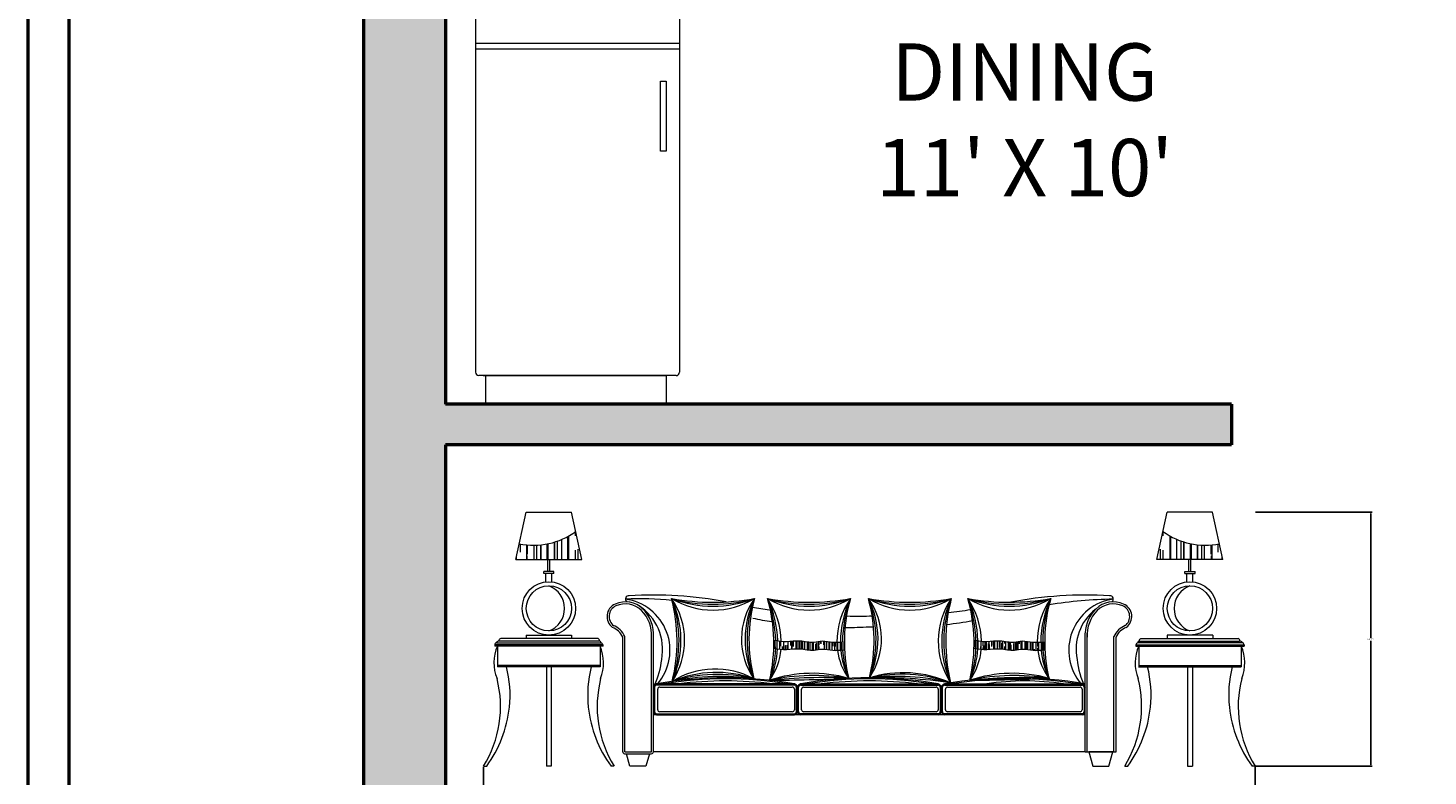
# Model space of a CAD drawing. Units: inches. Extents: x 1771 to 3025, y 319 to 889.
# Tile 31 of 35: x 2683 to 2854, y 714 to 805. Entities that reach past the tile are written whole.
import ezdxf

# ---------------------------------------------------------------- set-up
doc = ezdxf.new("R2010")
doc.units = ezdxf.units.IN
doc.header["$MEASUREMENT"] = 0
doc.set_wipeout_variables(frame=1)
for name, color, linetype, lineweight in [('A-ANNO-DIMS', 2, 'Continuous', 18), ('A-AREA-IDEN', 241, 'Continuous', 25), ('A-FURN', 8, 'Continuous', 18), ('A-WALL', 7, 'Continuous', 50), ('A-WALL-PATT', 254, 'Continuous', 13)]:
    doc.layers.add(name, color=color, linetype=linetype, lineweight=lineweight)
doc.styles.get("Standard").update_dxf_attribs({"font": 'arial.ttf'})
doc.dimstyles.get("Standard").update_dxf_attribs({"dimtxt": 0.18, "dimasz": 0.18, "dimexe": 0.18, "dimexo": 0.0625, "dimgap": 0.09, "dimtad": 0, "dimtih": 1, "dimtoh": 1, "dimdec": 4, "dimzin": 0, "dimdsep": 46, "dimtxsty": 'Standard', "dimcen": 0.09, "dimadec": 0, "dimazin": 0, "dimtfac": 1, "dimtdec": 4, "dimtofl": 0, "dimtmove": 0, "dimatfit": 3, "dimfxl": 1, "dimtolj": 1, "dimtzin": 0, "dimarcsym": 0})

# ---------------------------------------------------------------- blocks, each defined once
blk = doc.blocks.new('A$C301F3DA3')
for p, q in [((156.7, 1006), (206.7, 1236)), ((206.7, 1236), (427.8, 1236)), ((477.8, 1006), (427.8, 1236)), ((3275.4, 1006), (3325.4, 1236)), ((3546.5, 1236), (3325.4, 1236)), ((3596.5, 1006), (3546.5, 1236)), ((344.5, 1006), (344.5, 1090.3)), ((347, 1006), (347, 1091.1)), ((359.5, 1006), (359.5, 1095.2)), ((380.5, 1006), (380.5, 1103.5)), ((409.5, 1006), (409.5, 1117.6)), ((411, 1006), (411, 1118.4)), ((414, 1006), (414, 1120.1)), ((447.5, 1121.4), (447.5, 1141.6)), ((3305.7, 1121.4), (3305.7, 1141.6)), ((3339.2, 1006), (3339.2, 1120.1)), ((3342.2, 1006), (3342.2, 1118.4)), ((3343.7, 1006), (3343.7, 1117.6)), ((3372.7, 1006), (3372.7, 1103.5)), ((3393.7, 1006), (3393.7, 1095.2)), ((3406.2, 1006), (3406.2, 1091.1)), ((3408.7, 1006), (3408.7, 1090.3)), ((179.5, 1041.4), (179.5, 1081.1)), ((209.5, 1006), (209.5, 1076.8)), ((211.5, 1060.9), (211.5, 1076.6)), ((211.5, 1006), (211.5, 1023.4)), ((213, 1031.4), (213, 1076.5)), ((246.5, 1006), (246.5, 1075.2)), ((259.5, 1006), (259.5, 1075.6)), ((278, 1006), (278, 1073.4)), ((280, 1006), (280, 1077.1)), ((309.5, 1006), (309.5, 1081.6)), ((313.5, 1006), (313.5, 1082.4)), ((447.5, 1006), (447.5, 1051.4)), ((459.5, 1006), (459.5, 1056.4)), ((3293.7, 1006), (3293.7, 1056.4)), ((3305.7, 1006), (3305.7, 1051.4)), ((3439.7, 1006), (3439.7, 1082.4)), ((3443.7, 1006), (3443.7, 1081.6)), ((3473.2, 1006), (3473.2, 1077.1)), ((3475.2, 1006), (3475.2, 1073.4)), ((3493.7, 1006), (3493.7, 1075.6)), ((3506.7, 1006), (3506.7, 1075.2)), ((3540.2, 1031.4), (3540.2, 1076.5)), ((3541.7, 1060.9), (3541.7, 1076.6)), ((3541.7, 1006), (3541.7, 1023.4)), ((3543.7, 1006), (3543.7, 1076.8)), ((3573.7, 1041.4), (3573.7, 1081.1)), ((156.7, 1006), (477.8, 1006)), ((159.5, 1006), (159.5, 1019)), ((312.2, 948), (312.2, 1006)), ((322.2, 948), (322.2, 1006)), ((322.2, 948), (322.2, 1006)), ((477.5, 1006), (477.5, 1007.2)), ((3596.5, 1006), (3275.4, 1006)), ((3275.7, 1006), (3275.7, 1007.2)), ((3431, 948), (3431, 1006)), ((3431, 948), (3431, 1006)), ((3441, 948), (3441, 1006)), ((3593.7, 1006), (3593.7, 1019)), ((292.2, 938), (292.2, 948)), ((342.2, 948), (292.2, 948)), ((342.2, 938), (292.2, 938)), ((302.2, 896.9), (302.2, 938)), ((332.2, 896.9), (332.2, 938)), ((342.2, 938), (342.2, 948)), ((3411, 938), (3411, 948)), ((3411, 948), (3461, 948)), ((3411, 938), (3461, 938)), ((3421, 896.9), (3421, 938)), ((3451, 896.9), (3451, 938)), ((3461, 938), (3461, 948)), ((557.5, 620.8), (82.9, 620.8)), ((206.3, 637.8), (428.1, 637.8)), ((206.3, 637.8), (206.3, 620.8)), ((428.1, 637.8), (428.1, 620.8)), ((3195.6, 620.8), (3670.3, 620.8)), ((3546.9, 637.8), (3325, 637.8)), ((3325, 637.8), (3325, 620.8)), ((3546.9, 637.8), (3546.9, 620.8)), ((53.7, 590.8), (53.7, 584.4)), ((67.1, 584.4), (67.1, 484)), ((565.7, 608.8), (75.3, 608.8)), ((557.5, 608.8), (82.9, 608.8)), ((3187.5, 608.8), (3677.9, 608.8)), ((3195.6, 608.8), (3670.3, 608.8)), ((3686.1, 584.4), (3686.1, 484)), ((3699.5, 590.8), (3699.5, 584.4)), ((305.2, 484), (305.2, 0)), ((329.2, 484), (329.2, 0)), ((3424, 484), (3424, 0)), ((3448, 484), (3448, 0)), ((0, 0), (14.7, 0)), ((329.2, 0), (305.2, 0)), ((3424, 0), (3448, 0)), ((3753.2, 0), (3738.4, 0))]:
    blk.add_line(p, q)
for centre, radius in [((317.2, 767.8), 130), ((3436, 767.8), 130), ((317.2, 767.8), 110), ((3436, 767.8), 110)]:
    blk.add_circle(centre, radius)
for centre, radius, start, end in [((243.2, 1422.6), 347.4, 258.38286, 306.14668), ((3510, 1422.6), 347.4, 233.85332, 281.61714), ((276.7, 767.8), 117.2, 290.217, 69.783), ((3476.5, 767.8), 117.2, 110.217, 249.783), ((86.1, 609.2), 12.1, 105.22692, 181.3736), ((551.7, 609.3), 12.5, 357.63421, 66.98041), ((3201.5, 609.3), 12.5, 113.01959, 182.36579), ((3667.1, 609.2), 12.1, 358.6264, 74.77308), ((250.8, 503.3), 200.8, 156.16528, 202.38219), ((63.8, 591), 10.1, 100.6467, 181.11305), ((74, 595.7), 13.1, 84.28738, 156.7847), ((3679.2, 595.7), 13.1, 23.2153, 95.71262), ((3502.4, 503.3), 200.8, 337.61781, 23.83472), ((3689.4, 591), 10.1, 358.88695, 79.3533), ((-428.9, 346.4), 557.3, 353.82498, 14.29835), ((1063.3, 346.4), 557.3, 165.70165, 186.17502), ((2689.9, 346.4), 557.3, 353.82498, 14.29835), ((4182.1, 346.4), 557.3, 165.70165, 186.17502), ((-472, 290.4), 554.2, 328.39652, 14.25331), ((4225.2, 290.4), 554.2, 165.74669, 211.60348), ((-467.1, 350.3), 595.7, 323.98153, 353.84466), ((4220.2, 350.3), 595.7, 186.15534, 216.01847)]:
    blk.add_arc(centre, radius, start, end)
blk.add_wipeout([(3041.8, 0), (2963.5, 0), (2943.5, 70), (826.6, 70), (824.2, 65.5), (819.2, 61.4), (815.3, 60), (806.8, 60), (789.7, 0), (711.4, 0), (694.3, 60), (685.4, 60), (681.9, 61.7), (678.1, 65.9), (676.6, 70), (676.6, 628.7), (667.5, 644), (650.9, 661.4), (635.1, 671.5), (625.4, 676.3), (610.1, 693.4), (602.5, 710.5), (600.1, 728.4), (604.2, 751.4), (623, 778.5), (639.5, 788.9), (669, 798), (689.6, 799.7), (696.6, 800), (691.2, 806.8), (690.2, 814.9), (693.8, 823.2), (701.1, 828), (705.9, 828.8), (865.5, 832), (984.1, 825.9), (1111.6, 811), (1170.7, 801.2), (1180.3, 799.4), (1231.4, 803.5), (1293.2, 811.6), (1317.6, 815.8), (1310.3, 786.3), (1307.6, 774.2), (1389.8, 761.2), (1393.6, 767.5), (1388.1, 790.9), (1381.5, 815.8), (1418.2, 809.7), (1480.9, 802.2), (1546.1, 798.2), (1588.9, 797.6), (1683.4, 802), (1730, 807.2), (1784.7, 815.8), (1774.6, 776.7), (1767.8, 744), (1769.2, 730.8), (1890.2, 730.7), (1884.7, 761.4), (1877, 795.8), (1871.7, 815.8), (1919.1, 808.2), (1966.4, 802.7), (2026, 798.6), (2073.3, 797.6), (2145.9, 799.9), (2221.5, 807.4), (2273.8, 815.4), (2267.3, 783.6), (2260.5, 748.2), (2369.1, 762), (2361.7, 794), (2355.9, 815.8), (2402.1, 808.4), (2442.8, 803.5), (2477.3, 800.5), (2535.4, 797.9), (2572.4, 797.9), (2610.4, 806.1), (2648.6, 812), (2670.2, 815.1), (2740.7, 823.3), (2819.6, 829.3), (2905.4, 832.2), (2981.5, 831.5), (3045.3, 828.6), (3053.9, 827.3), (3059.6, 822.9), (3062.8, 816.3), (3062.9, 810.1), (3060.6, 804.3), (3056.6, 800), (3070.6, 799.5), (3085.9, 797.7), (3105.1, 792.4), (3120.7, 785.3), (3134.4, 774.5), (3143.7, 762.3), (3150.7, 746.2), (3153, 725.9), (3150.1, 708.7), (3142.9, 693.1), (3133.2, 681), (3126.6, 675.3), (3114.9, 669.8), (3100.2, 659.6), (3082.1, 638.7), (3076.6, 628.7), (3076.6, 70), (3061.8, 70)])
for p, q in [((3056.6, 800), (3056.6, 799.5)), ((676.6, 70), (676.6, 628.7)), ((686.6, 70), (686.6, 630.8)), ((816.6, 70), (816.6, 647.2)), ((826.6, 70), (826.6, 627.7)), ((2926.6, 70), (2926.6, 647.2)), ((2936.6, 70), (2936.6, 647.2)), ((3066.6, 70), (3066.6, 630.8)), ((3076.6, 70), (3076.6, 628.7)), ((580.7, 590.8), (53.7, 590.8)), ((580.7, 584.4), (53.7, 584.4)), ((61.9, 600.9), (572.5, 600.9)), ((566.3, 584.4), (566.3, 484)), ((579.7, 590.8), (579.7, 584.4)), ((3172.5, 590.8), (3699.5, 590.8)), ((3172.5, 584.4), (3699.5, 584.4)), ((3173.5, 590.8), (3173.5, 584.4)), ((3691.3, 600.9), (3180.7, 600.9)), ((3186.9, 584.4), (3186.9, 484)), ((567.3, 490), (67.1, 490)), ((567.3, 484), (67.1, 484)), ((3185.9, 490), (3686.1, 490)), ((3185.9, 484), (3686.1, 484)), ((826.6, 400), (826.6, 265)), ((1511.6, 400), (841.6, 400)), ((1511.2, 395), (841.6, 395)), ((846.6, 275), (846.6, 375)), ((856.6, 385), (1501.6, 385)), ((1511.6, 375), (1511.6, 275)), ((1526.6, 265), (1526.6, 385)), ((1526.6, 265), (1526.6, 385)), ((1531.6, 265.4), (1531.6, 384.6)), ((1541.6, 400), (2211.6, 400)), ((1542, 395), (2211.2, 395)), ((1546.6, 275), (1546.6, 375)), ((1556.6, 385), (2201.6, 385)), ((2211.6, 375), (2211.6, 275)), ((2221.6, 384.6), (2221.6, 265.4)), ((2226.6, 265), (2226.6, 385)), ((2226.6, 385), (2226.6, 265)), ((2231.6, 265.4), (2231.6, 384.6)), ((2241.6, 400), (2911.6, 400)), ((2242, 395), (2911.2, 395)), ((2246.6, 275), (2246.6, 375)), ((2256.6, 385), (2901.6, 385)), ((2911.6, 375), (2911.6, 275)), ((2921.6, 384.6), (2921.6, 265.4)), ((1511.6, 250), (826.6, 250)), ((2926.6, 250), (826.6, 250)), ((841.6, 250), (1511.6, 250)), ((842, 255), (1511.6, 255)), ((1501.6, 265), (856.6, 265)), ((2211.6, 255), (1542, 255)), ((2201.6, 265), (1556.6, 265)), ((2911.2, 255), (2242, 255)), ((2901.6, 265), (2256.6, 265)), ((686.6, 70), (816.6, 70)), ((2926.6, 70), (826.6, 70)), ((2926.6, 70), (3076.6, 70)), ((3061.8, 70), (2943.5, 70)), ((2943.5, 70), (2963.5, 0)), ((3041.8, 0), (3061.8, 70)), ((633.4, 0), (618.7, 0)), ((685.4, 60), (815.3, 60)), ((711.4, 0), (694.3, 60)), ((789.7, 0), (711.4, 0)), ((806.8, 60), (789.7, 0)), ((2963.5, 0), (3041.8, 0)), ((3119.8, 0), (3134.5, 0))]:
    blk.add_line(p, q)
at = {"ltscale": 0.1}
for p, q in [((1414.4, 573.7), (1414.4, 606.7)), ((1418.8, 573), (1418.8, 612.1)), ((1420.6, 572.7), (1420.6, 580.7)), ((1427.8, 571.6), (1427.8, 610.7)), ((1440.6, 576.7), (1440.6, 609)), ((1441.2, 569.8), (1441.2, 608.9)), ((1445.4, 583.3), (1445.4, 608.4)), ((1454.6, 568.5), (1454.6, 582.7)), ((1460.6, 568.1), (1460.6, 607.2)), ((1468, 606.7), (1468, 607)), ((1468, 567.8), (1468, 586.7)), ((1472, 603.3), (1472, 606.9)), ((1472, 567.8), (1472, 588.3)), ((1480.6, 568.1), (1480.6, 588.7)), ((1481.4, 568.1), (1481.4, 607.3)), ((1494.8, 586.7), (1494.8, 608.3)), ((1498.6, 569.5), (1498.6, 608.3)), ((1500.6, 569.7), (1500.6, 608.8)), ((1508.2, 582.7), (1508.2, 609.5)), ((1520.6, 571.3), (1520.6, 610.4)), ((1521.6, 571.4), (1521.6, 610.5)), ((1525.2, 571.5), (1525.2, 610.6)), ((1535, 571.6), (1535, 610.7)), ((1540.6, 571.3), (1540.6, 610.4)), ((1548.4, 570.6), (1548.4, 609.6)), ((1551.8, 570.1), (1551.8, 609.2)), ((1560.6, 568.8), (1560.6, 607.9)), ((1561.8, 568.6), (1561.8, 607.7)), ((1575.2, 566.4), (1575.2, 605.5)), ((1578.4, 565.9), (1578.4, 605)), ((1580.6, 565.6), (1580.6, 604.7)), ((1588.6, 564.6), (1588.6, 603.7)), ((1600.6, 564), (1600.6, 603.1)), ((1602, 564), (1602, 590.7)), ((1605, 568.3), (1605, 603.3)), ((1615.4, 565.2), (1615.4, 594.7)), ((1620.6, 566.1), (1620.6, 600.7)), ((1628.8, 567.7), (1628.8, 606.9)), ((1631.6, 588.3), (1631.6, 607.4)), ((1631.6, 568.2), (1631.6, 581.7)), ((1640.6, 596.7), (1640.6, 608.8)), ((1642.2, 594.7), (1642.2, 609)), ((1655.6, 590.7), (1655.6, 609.3)), ((1655.6, 570.2), (1655.6, 570.7)), ((1658.2, 608.3), (1658.2, 609.1)), ((1658.2, 570), (1658.2, 601.7)), ((1660.6, 569.8), (1660.6, 608.9)), ((1669, 568.8), (1669, 607.9)), ((1680.6, 566.9), (1680.6, 606)), ((1682.4, 570.7), (1682.4, 605.7)), ((1684.8, 566.2), (1684.8, 605.3)), ((1695.8, 566.7), (1695.8, 603.7)), ((1700.6, 584.7), (1700.6, 603.2)), ((1700.6, 564.1), (1700.6, 564.7)), ((1709.2, 563.6), (1709.2, 602.7)), ((1711.4, 581.7), (1711.4, 602.7)), ((1711.4, 563.6), (1711.4, 566.7)), ((1720.6, 563.7), (1720.6, 602.8)), ((1722.6, 563.7), (1722.6, 602.9)), ((1736, 564.6), (1736, 603.8)), ((1738, 601.7), (1738, 603.9)), ((1738, 564.8), (1738, 586.7)), ((1740.6, 565), (1740.6, 604.2)), ((1749.4, 565.9), (1749.4, 598.7)), ((2392.6, 573.1), (2392.6, 610.7)), ((2400.6, 571.9), (2400.6, 610.9)), ((2403, 571.5), (2403, 610.6)), ((2406, 571.1), (2406, 610.1)), ((2419.4, 569.4), (2419.4, 582.7)), ((2420.6, 569.2), (2420.6, 608.3)), ((2429.6, 583.5), (2429.6, 607.5)), ((2429.6, 568.4), (2429.6, 576.9)), ((2432.8, 606.7), (2432.8, 607.3)), ((2432.8, 568.2), (2432.8, 586.7)), ((2440.6, 567.9), (2440.6, 607)), ((2446.2, 567.8), (2446.2, 606.9)), ((2456.2, 603.5), (2456.2, 607.3)), ((2456.2, 568.1), (2456.2, 596.9)), ((2459.6, 586.7), (2459.6, 607.5)), ((2460.6, 568.4), (2460.6, 592.7)), ((2473, 582.7), (2473, 608.6)), ((2480.6, 588.7), (2480.6, 609.3)), ((2482.8, 570.4), (2482.8, 609.5)), ((2486.4, 570.7), (2486.4, 609.8)), ((2499.8, 571.5), (2499.8, 610.6)), ((2500.6, 571.5), (2500.6, 610.7)), ((2509.4, 576.9), (2509.4, 610.7)), ((2513.2, 571.4), (2513.2, 610.5)), ((2520.6, 570.8), (2520.6, 600.7)), ((2526.6, 570.1), (2526.6, 609.1)), ((2536, 596.9), (2536, 607.7)), ((2536, 568.6), (2536, 581.9)), ((2540, 568), (2540, 607)), ((2540.6, 576.7), (2540.6, 606.9)), ((2553.4, 565.8), (2553.4, 604.9)), ((2560.6, 564.9), (2560.6, 604)), ((2562.6, 564.7), (2562.6, 601.9)), ((2566.8, 564.3), (2566.8, 590.7)), ((2580.2, 564.2), (2580.2, 594.7)), ((2580.6, 564.2), (2580.6, 603.3)), ((2589.2, 565.2), (2589.2, 604.3)), ((2593.6, 565.9), (2593.6, 605.1)), ((2600.6, 567.2), (2600.6, 606.4)), ((2607, 594.7), (2607, 607.6)), ((2615.8, 569.8), (2615.8, 608.9)), ((2620.4, 590.7), (2620.4, 609.3)), ((2620.4, 570.2), (2620.4, 570.7)), ((2620.6, 570.2), (2620.6, 609.3)), ((2633.8, 570), (2633.8, 609)), ((2640.6, 569.2), (2640.6, 608.3)), ((2642.4, 569), (2642.4, 608)), ((2647.2, 570.7), (2647.2, 607.3)), ((2660.6, 566), (2660.6, 605.1)), ((2660.6, 566.7), (2660.6, 605.1)), ((2669, 564.8), (2669, 603.8)), ((2674, 564.2), (2674, 603.3)), ((2680.6, 563.8), (2680.6, 568.7)), ((2687.4, 563.6), (2687.4, 602.7)), ((2695.6, 581.9), (2695.6, 602.8)), ((2695.6, 563.7), (2695.6, 575.3)), ((2700.6, 564.7), (2700.6, 603.1)), ((2700.8, 563.9), (2700.8, 603.1)), ((2714.2, 565), (2714.2, 598.7)), ((2720.6, 565.6), (2720.6, 604.8)), ((2722.2, 601.9), (2722.2, 604.9)), ((2722.2, 565.8), (2722.2, 595.3)), ((2727.6, 566.4), (2727.6, 602.7))]:
    blk.add_line(p, q, dxfattribs=at)
at = {"ltscale": 0.2}
for p, q in [((831.6, 384.6), (831.6, 265.4)), ((1521.6, 265.4), (1521.6, 384.6))]:
    blk.add_line(p, q, dxfattribs=at)
for centre, radius, start, end in [((705.9, 812.9), 15.9, 82.92998, 233.99863), ((826.9, -1080.6), 1912.9, 79.35353, 93.56712), ((2926.5, -1083.7), 1916.1, 86.44665, 100.89711), ((3047.3, 812.9), 15.9, 306.00137, 97.07002), ((666.4, 728.4), 66.3, 113.9424, 233.11156), ((666.4, 728.4), 56.3, 113.9424, 233.11156), ((689.6, 677.8), 121.9, 45.5351, 114.26403), ((689.6, 677.8), 111.9, 45.5351, 114.26403), ((647.8, 638.7), 169.2, 356.50689, 44.75015), ((647.8, 638.7), 179.2, 356.50689, 44.75015), ((118.5, 608.8), 822.4, 346.1538, 14.5736), ((1116, 1923.3), 1125.7, 259.68325, 280.31675), ((2062.3, 614.6), 771.4, 164.88081, 194.22903), ((1820.4, 3753.3), 3022.9, 260.23295, 261.81056), ((611.7, 598.3), 800, 346.95646, 15.77378), ((1583.1, 1923.3), 1125.7, 259.68325, 280.31675), ((2517.6, 605.2), 762.6, 163.96966, 193.48898), ((2073.3, 1923.3), 1125.7, 259.68325, 280.31675), ((1147.1, 613.7), 752.3, 345.86352, 15.58525), ((3098.6, 604.6), 850.3, 165.62179, 193.5679), ((1932.8, 3753.3), 3022.9, 276.22345, 278.29852), ((2556.6, 1923.4), 1125.7, 259.73156, 280.36506), ((1586.1, 598.3), 800, 346.95646, 15.77378), ((3493.3, 605.3), 763.9, 163.98353, 193.47734), ((3105.4, 638.7), 179.2, 135.24985, 176.50689), ((3105.4, 638.7), 169.2, 135.24985, 183.49311), ((3063.6, 677.8), 121.9, 65.73597, 134.4649), ((3063.6, 677.8), 111.9, 65.73597, 134.4649), ((3086.8, 728.4), 56.3, 306.88844, 66.0576), ((3086.8, 728.4), 66.3, 306.88844, 66.0576), ((593.4, 589.7), 101.9, 23.83547, 68.81673), ((1820.4, 3753.3), 3022.9, 269.03014, 271.06523), ((1932.8, 3753.3), 3022.9, 268.93477, 269.19298), ((3159.8, 589.7), 101.9, 112.01062, 156.16453), ((593.4, 589.7), 91.9, 24.95202, 68.81673), ((3159.8, 589.7), 91.9, 111.18327, 155.04798), ((561.8, 599.3), 9.8, 9.61841, 76.53695), ((382.6, 503.3), 200.8, 337.61781, 23.83472), ((562.8, 585.5), 17.7, 17.55797, 60.68227), ((3370.5, 503.3), 200.8, 156.16528, 202.38219), ((3190.4, 585.5), 17.7, 119.31773, 162.44203), ((3191.3, 599.3), 9.8, 103.46305, 170.38159), ((1106.4, 290.4), 554.2, 165.74669, 211.60348), ((1176.6, -1455.4), 1885.4, 79.76537, 100.23463), ((1150.7, -658.8), 1096, 81.40397, 102.31547), ((1256.5, 13610.3), 13193.2, 270.58435, 272.25734), ((1876.6, -1455.4), 1885.4, 79.76537, 100.23463), ((1933.3, -1830.3), 2260.9, 81.38364, 91.43687), ((2584.1, -1540.1), 1970.1, 79.98833, 100.01167), ((2230.8, 13610.3), 13193.2, 270.58435, 272.25734), ((2646.8, 290.4), 554.2, 328.39652, 14.25331), ((844.1, 382.5), 17.7, 98.1301, 171.8699), ((844.1, 382.5), 12.7, 101.3731, 171.8699), ((856.6, 375), 10, 90, 180), ((1501.6, 375), 10, 0, 90), ((1509.1, 382.5), 12.7, 9.60357, 81.8699), ((1509.1, 382.5), 17.7, 8.1301, 81.8699), ((1544.1, 382.5), 17.7, 98.1301, 171.8699), ((1544.1, 382.5), 12.7, 99.60357, 170.39643), ((1556.6, 375), 10, 90, 180), ((2201.6, 375), 10, 0, 90), ((2209.1, 382.5), 12.7, 9.60357, 81.8699), ((2209.1, 382.5), 17.7, 8.1301, 81.8699), ((2244.1, 382.5), 17.7, 98.1301, 171.8699), ((2244.1, 382.5), 12.7, 98.1301, 170.39643), ((2256.6, 375), 10, 90, 180), ((2901.6, 375), 10, 0, 90), ((2909.1, 382.5), 12.7, 9.60357, 80.39643), ((2909.1, 382.5), 17.7, 8.1301, 81.8699), ((1101.5, 350.3), 595.7, 186.15534, 216.01847), ((856.6, 275), 10, 180, 270), ((1501.6, 275), 10, 270, 0), ((1556.6, 275), 10, 180, 270), ((2201.6, 275), 10, 270, 0), ((2256.6, 275), 10, 180, 270), ((2901.6, 275), 10, 270, 0), ((2651.7, 350.3), 595.7, 323.98153, 353.84466), ((844.1, 267.5), 17.7, 188.1301, 261.8699), ((844.1, 267.5), 12.7, 189.60357, 260.39643), ((1509.1, 267.5), 12.7, 278.1301, 351.8699), ((1509.1, 267.5), 17.7, 278.1301, 351.8699), ((1544.1, 267.5), 17.7, 188.1301, 261.8699), ((1544.1, 267.5), 12.7, 188.1301, 261.8699), ((2209.1, 267.5), 12.7, 278.1301, 350.39643), ((2209.1, 267.5), 17.7, 278.1301, 351.8699), ((2244.1, 267.5), 17.7, 188.1301, 261.8699), ((2244.1, 267.5), 12.7, 189.60357, 261.8699), ((2909.1, 267.5), 12.7, 278.1301, 350.39643), ((2909.1, 267.5), 17.7, 278.1301, 351.8699), ((689.4, 72.4), 13, 190.46913, 252.22973), ((812.4, 74.7), 15, 281.33001, 341.83756)]:
    blk.add_arc(centre, radius, start, end)
for centre, radius, start, end in [((760.4, -701.1), 1515.6, 84.07641, 92.659), ((655.5, 564.2), 251.1, 319.40416, 82.09148), ((615.4, 566.9), 255.3, 349.39262, 57.21951), ((478.9, 611.1), 481.1, 335.55638, 25.17102), ((347.1, 610.3), 603.3, 340.81637, 19.91104), ((617, 612), 360.5, 326.31194, 34.41547), ((1116, 1147.7), 388.4, 238.72737, 301.27263), ((1116, 1532.7), 744.8, 254.29016, 285.61296), ((1116.1, 1337.7), 559.4, 249.04787, 290.9906), ((1594, 618.2), 339.8, 144.44675, 214.66309), ((1723.9, 617.2), 452.3, 153.95498, 205.15486), ((1847.8, 616.2), 566.5, 159.37514, 199.7347), ((757.4, 589.8), 663.8, 1.89953, 19.9071), ((904.2, 593.4), 526.6, 1.83653, 24.977), ((1057.3, 597.5), 390.8, 1.55805, 33.94797), ((1583.1, 1147.7), 388.4, 238.72737, 301.27263), ((1583.2, 1532.7), 744.8, 254.29016, 285.61296), ((1583.2, 1337.7), 559.4, 249.04787, 290.9906), ((2089.5, 604.3), 371, 145.24271, 180.23552), ((2233.6, 600.8), 497.7, 154.4139, 179.66501), ((2371.5, 597.7), 626, 159.61394, 179.36153), ((2073.3, 1147.7), 388.4, 238.72737, 301.27263), ((2073.4, 1532.7), 744.8, 254.29016, 285.61296), ((1604, 619.4), 332, 325.19263, 36.25614), ((1356.4, 616.3), 552.6, 340.29034, 21.15843), ((1477.2, 617.8), 441.4, 334.80604, 26.64273), ((2073.4, 1337.7), 559.4, 249.04787, 290.9906), ((2583.5, 608.3), 371.9, 146.08399, 213.1057), ((2726, 607.2), 497, 155.19256, 203.99713), ((2862.3, 606.3), 623.6, 160.37041, 198.81928), ((2557.2, 1147.9), 388.4, 238.77569, 301.32093), ((1731.8, 589.8), 663.8, 1.89953, 19.9071), ((1878.6, 593.4), 526.6, 1.83653, 24.977), ((2031.7, 597.5), 390.8, 1.55805, 33.94797), ((2556.9, 1532.9), 744.8, 254.33859, 285.66141), ((2557.2, 1337.9), 559.4, 249.09653, 291.03924), ((3065, 604.3), 372, 145.29362, 180.23636), ((3209.5, 600.8), 499.2, 154.45299, 179.66602), ((3347.8, 597.7), 627.9, 159.64574, 179.36278), ((3116.2, -1577.3), 2390.8, 91.27111, 98.78687), ((3097.7, 564.2), 251.1, 97.90852, 220.59584), ((3129.1, 568.5), 247.1, 128.48308, 191.34035), ((1756.4, 2902), 2227.1, 258.42921, 260.84468), ((1995, 2902), 2227.1, 276.64183, 279.91471), ((1756.4, 2902), 2227.1, 270.09381, 273.07097), ((1995, 2902), 2227.1, 266.92903, 267.47072), ((902.9, 592.1), 518.2, 340.3477, 357.85991), ((1016.3, 594.9), 414.5, 334.69408, 356.73006), ((1135.5, 598), 312.7, 324.80426, 354.71594), ((2016.9, 603.5), 298.4, 187.6695, 216.19187), ((2130.5, 600.8), 394.6, 185.24411, 206.08232), ((2238.4, 598.3), 492.9, 183.79515, 200.29326), ((1877.3, 592.1), 518.2, 340.3477, 357.85991), ((1990.7, 594.9), 414.5, 334.69408, 356.73006), ((2109.9, 598), 312.7, 324.80426, 354.71594), ((2991.3, 603.5), 298.4, 187.6695, 216.19187), ((3104.9, 600.8), 394.6, 185.24411, 206.08232), ((3212.8, 598.3), 492.9, 183.79515, 200.29326), ((468.9, 563.6), 399.8, 334.99578, 353.7174), ((3284.3, 563.6), 399.8, 186.2826, 206.53978), ((1176.6, -1429.1), 1854.1, 80.58034, 99.41966), ((1126.7, 81.6), 391.4, 61.31825, 122.4012), ((1138.5, -278.6), 725.3, 76.04293, 107.78495), ((1132.5, -88.7), 544.9, 70.60179, 113.1041), ((1176.6, -1342.3), 1757.3, 82.5085, 97.4915), ((1599, -199.4), 651.3, 74.21866, 108.62302), ((1646.2, -2030.8), 2461.8, 87.00101, 95.95019), ((1608.6, -583.8), 1025.1, 80.66015, 102.16113), ((1876.6, -1429.1), 1854.1, 80.58034, 99.41966), ((1876.6, -1429.1), 1844.1, 82.68708, 97.31292), ((2041.7, -102.7), 557.6, 65.60138, 107.21913), ((2031.9, -256.9), 704.2, 70.15873, 102.74025), ((2004.4, -699.8), 1137, 76.44399, 96.45498), ((2584.1, -1521.2), 1946.2, 80.80656, 99.19344), ((2573.4, -199.4), 651.3, 74.21866, 108.62302), ((2620.6, -2030.8), 2461.8, 87.00101, 95.95019), ((2583, -583.8), 1025.1, 80.66015, 102.16113), ((2634.1, -753.4), 1168.4, 80.80901, 99.19099)]:
    blk.add_arc(centre, radius, start, end, dxfattribs=at)
for points in [[(1411.2, 613.3), (1432, 609.9), (1474.4, 603.1), (1540.1, 616.4), (1597.7, 597.2), (1650.5, 614.1), (1699.8, 599.6), (1736.2, 603.6), (1755.3, 605.7)], [(2385.5, 613.3), (2406.4, 609.9), (2448.8, 603.1), (2514.5, 616.4), (2572, 597.2), (2624.9, 614.1), (2674.2, 599.6), (2710.6, 603.6), (2729.6, 605.7)], [(1411.5, 574.2), (1432.4, 570.8), (1474.8, 564), (1540.5, 577.3), (1598, 558.1), (1650.9, 575), (1700.2, 560.5), (1736.6, 564.5), (1755.6, 566.6)], [(2385.9, 574.2), (2406.8, 570.8), (2449.2, 564), (2514.8, 577.3), (2572.4, 558.1), (2625.2, 575), (2674.5, 560.5), (2711, 564.5), (2730, 566.6)]]:
    blk.add_open_spline(points, degree=3, knots=[0, 0, 0, 0, 62.941123, 128.023226, 196.918691, 236.354413, 288.676993, 345.703861, 345.703861, 345.703861, 345.703861])
blk = doc.blocks.new('A$C43BC2F3A')
for p, q in [((0, 1490.5), (0, 93.5)), ((10, 1500), (590, 1500)), ((600, 1490), (600, 93.5)), ((590, 83.5), (10.3, 83.5)), ((22.6, 83.5), (561, 83.5)), ((30.8, 0), (30.8, 83.5)), ((561, 83.5), (561, 0)), ((561, 0), (30.8, 0))]:
    blk.add_line(p, q)
for points in [[(561, 1344.2), (561, 1188.3), (544.3, 1188.3), (544.3, 1344.2)], [(561, 949), (561, 743), (544.3, 743), (544.3, 949)]]:
    blk.add_lwpolyline(points, close=True)
for points in [[(600, 1060.3), (0, 1060.3)], [(600, 1043.6), (0, 1043.6)]]:
    blk.add_lwpolyline(points)
for centre, radius, start, end in [((10, 1490), 10, 90, 180), ((590, 1490), 10, 0, 90), ((10.5, 94), 10.5, 182.8791, 268.8051), ((590, 93.5), 10, 270, 0)]:
    blk.add_arc(centre, radius, start, end)
blk = doc.blocks.new('*D46')
at = {"layer": 'A-ANNO-DIMS', "color": 0, "lineweight": -2, "transparency": 16777216}
for p, q in [((2738.34, 715.17), (2738.34, 700.92)), ((2832.56, 715.17), (2832.56, 700.92)), ((2738.52, 701.1), (2784.55, 701.1)), ((2832.38, 701.1), (2786.36, 701.1))]:
    blk.add_line(p, q, dxfattribs=at)
at = {"layer": 'A-ANNO-DIMS', "color": 0, "transparency": 16777216}
for points in [[(2738.52, 701.13), (2738.52, 701.07), (2738.34, 701.1)], [(2832.38, 701.13), (2832.38, 701.07), (2832.56, 701.1)]]:
    blk.add_solid(points, dxfattribs=at)
at = {"layer": 'Defpoints', "color": 0, "transparency": 16777216}
for p in [(2738.34, 715.24), (2832.56, 715.24), (2832.56, 701.1)]:
    blk.add_point(p, dxfattribs=at)
at = {"layer": 'A-ANNO-DIMS', "color": 0, "transparency": 16777216, "insert": (2785.45, 701.1), "char_height": 0.18, "attachment_point": 5}
blk.add_mtext('\\A1;SOFA 94 TYP.', dxfattribs=at)
blk = doc.blocks.new('*D47')
at = {"layer": 'A-ANNO-DIMS', "color": 0, "lineweight": -2, "transparency": 16777216}
for p, q in [((2832.63, 746.27), (2846.88, 746.27)), ((2846.7, 746.09), (2846.7, 730.93)), ((2846.7, 715.42), (2846.7, 730.57)), ((2832.63, 715.24), (2846.88, 715.24))]:
    blk.add_line(p, q, dxfattribs=at)
at = {"layer": 'A-ANNO-DIMS', "color": 0, "transparency": 16777216}
for points in [[(2846.67, 746.09), (2846.73, 746.09), (2846.7, 746.27)], [(2846.67, 715.42), (2846.73, 715.42), (2846.7, 715.24)]]:
    blk.add_solid(points, dxfattribs=at)
at = {"layer": 'Defpoints', "color": 0, "transparency": 16777216}
for p in [(2832.56, 746.27), (2846.7, 746.27), (2832.56, 715.24)]:
    blk.add_point(p, dxfattribs=at)
at = {"layer": 'A-ANNO-DIMS', "color": 0, "transparency": 16777216, "insert": (2846.7, 730.75), "char_height": 0.18, "attachment_point": 5}
blk.add_mtext('\\A1;31 TYP.', dxfattribs=at)

msp = doc.modelspace()

# ---------------------------------------------------------------- hatches: boundary and pattern name
at = {"layer": 'A-WALL-PATT'}
h = msp.add_hatch(color=256, dxfattribs=at)
h.dxf.hatch_style = 1
h.paths.add_polyline_path([(2870.68, 879.48), (2892.73, 879.48), (2892.73, 889.48), (2842.68, 889.48), (2842.68, 879.48), (2865.68, 879.48), (2865.68, 831.48), (2870.68, 831.48)])
h.paths.add_polyline_path([(2983.64, 889.48), (2940.73, 889.48), (2940.73, 879.48), (2961.68, 879.48), (2961.68, 795.48), (2865.68, 795.48), (2865.68, 759.48), (2865.68, 665.48), (2870.68, 665.48), (2870.68, 712.85), (2870.68, 790.48), (2978.68, 790.48), (2978.68, 795.48), (2966.68, 795.48), (2966.68, 879.48), (2983.64, 879.48)])
h.paths.add_polyline_path([(3024.68, 889.48), (3001.64, 889.48), (3001.64, 879.48), (3014.68, 879.48), (3014.68, 790.48), (3014.68, 769.46), (3024.68, 769.46)])
h.paths.add_polyline_path([(3024.68, 721.46), (3014.68, 721.46), (3014.68, 670.48), (2906.68, 670.48), (2906.68, 665.48), (2925.68, 665.48), (2925.68, 653.48), (2930.68, 653.48), (2930.68, 665.48), (3014.68, 665.48), (3014.68, 650.02), (3024.68, 650.02)])
h.paths.add_polyline_path([(3024.68, 632.02), (3014.68, 632.02), (3014.68, 617.48), (2925.68, 617.48), (2906.68, 617.48), (2906.68, 612.48), (3014.68, 612.48), (3014.68, 581.96), (3024.68, 581.96)])
h.paths.add_polyline_path([(3024.68, 533.96), (3014.68, 533.96), (3014.68, 480.48), (2870.68, 480.48), (2870.68, 617.48), (2860.68, 617.48), (2860.68, 544.48), (2769.68, 544.48), (2769.68, 534.48), (2860.68, 534.48), (2860.68, 470.48), (3014.68, 470.48), (3014.68, 453.61), (3024.68, 453.61)])
h.paths.add_polyline_path([(3024.68, 405.61), (3014.68, 405.61), (3014.68, 394.48), (2860.68, 394.48), (2860.68, 384.48), (3024.68, 384.48)])
h.paths.add_polyline_path([(2733.68, 643.43), (2723.68, 643.43), (2723.68, 534.48), (2733.68, 534.48)])
h.paths.add_polyline_path([(2733.68, 754.48), (2829.68, 754.48), (2829.68, 759.48), (2733.68, 759.48), (2733.68, 843.44, -0.008336), (2732.38, 843.48), (2723.68, 843.48), (2723.68, 691.43), (2733.68, 691.43)])
h.paths.add_polyline_path([(2794.68, 889.48), (2723.68, 889.48), (2723.68, 879.48), (2794.68, 879.48)])

# ---------------------------------------------------------------- linework, layer by layer
at = {"layer": 'A-WALL'}
for p, q in [((2682.68, 889.48), (2682.68, 534.48)), ((2687.68, 879.48), (2687.68, 534.48)), ((2723.68, 843.48), (2723.68, 534.48)), ((2733.68, 843.48), (2733.68, 759.48)), ((2829.68, 759.48), (2733.68, 759.48)), ((2829.68, 759.48), (2829.68, 754.48)), ((2829.68, 754.48), (2733.68, 754.48)), ((2733.68, 754.48), (2733.68, 534.48))]:
    msp.add_line(p, q, dxfattribs=at)

# ---------------------------------------------------------------- block references
at = {"layer": 'A-FURN', "xscale": 0.0415387277892195, "yscale": 0.0415387277892195, "zscale": 0.0415387277892195}
msp.add_blockref('A$C43BC2F3A', (2737.33, 759.48), dxfattribs=at)

# ---------------------------------------------------------------- texts
at = {"layer": 'A-AREA-IDEN', "insert": (2761.69, 803.53), "char_height": 7, "attachment_point": 1}
msp.add_mtext_dynamic_manual_height_columns("\\pxqc;DINING \\P11' X 10'", width=85.4611, gutter_width=1, heights=[0], dxfattribs=at)

# ---------------------------------------------------------------- next in the draw order: block references
at = {"layer": 'A-FURN', "xscale": 0.0251055470835414, "yscale": 0.0251055470835414, "zscale": 0.0251055470835414}
msp.add_blockref('A$C301F3DA3', (2738.34, 715.24), dxfattribs=at)

# ---------------------------------------------------------------- next in the draw order: dimensions: what is measured, and where the dimension line sits
at = {"layer": 'A-ANNO-DIMS'}
dim = msp.add_linear_dim(base=(2846.7, 746.27), p1=(2832.56, 715.24), p2=(2832.56, 746.27), angle=90, text='<> TYP.', dimstyle='Standard', override={"dimdec": 0, "dimrnd": 0, "dimzin": 0, "dimlunit": 2}, dxfattribs=at)
dim.commit()
dim.dimension.update_dxf_attribs({"geometry": '*D47', "text_midpoint": (2846.7, 730.75)})
dim = msp.add_linear_dim(base=(2832.56, 701.1), p1=(2738.34, 715.24), p2=(2832.56, 715.24), text='SOFA <> TYP.', dimstyle='Standard', override={"dimdec": 0, "dimrnd": 0, "dimzin": 0, "dimlunit": 2}, dxfattribs=at)
dim.commit()
dim.dimension.update_dxf_attribs({"geometry": '*D46', "text_midpoint": (2785.45, 701.1)})

doc.saveas('drawing.dxf')
